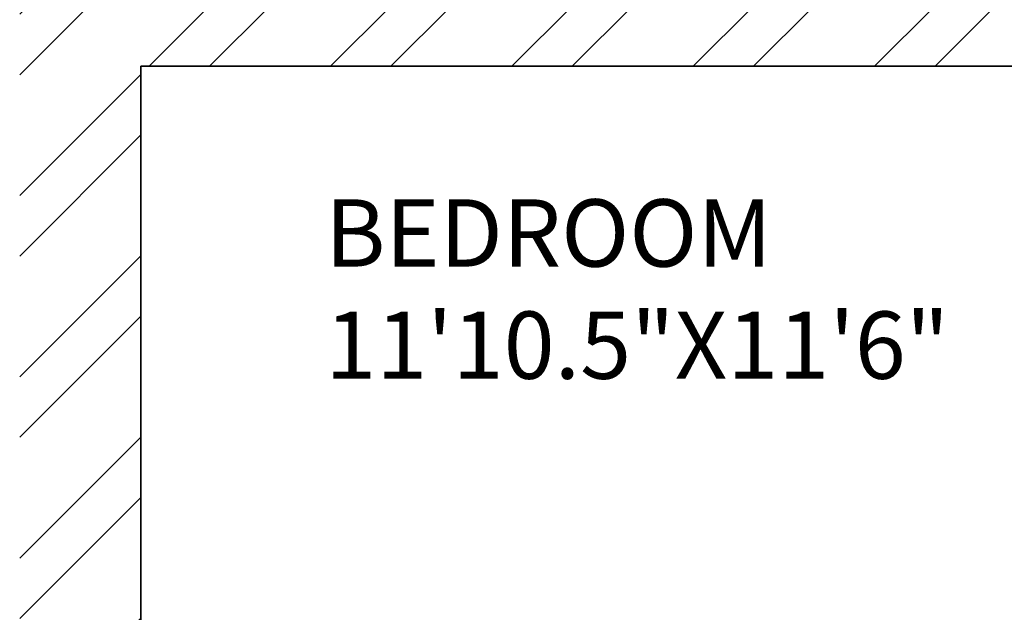
# Model space of a CAD drawing. Units: inches. Extents: x 2120 to 4013, y 1390 to 3019.
# Tile 18 of 59: x 2716 to 2789, y 1688 to 1732. Entities that reach past the tile are written whole.
import ezdxf

# ---------------------------------------------------------------- set-up
doc = ezdxf.new("R2010")
doc.units = ezdxf.units.IN
for name, color, linetype, lineweight in [('A-AREA-IDEN', 7, 'Continuous', 18), ('A-WALL', 7, 'Continuous', 35), ('A-WALL-PATT', 252, 'Continuous', 13)]:
    doc.layers.add(name, color=color, linetype=linetype, lineweight=lineweight)
doc.styles.get("Standard").update_dxf_attribs({"font": 'arial.ttf'})

msp = doc.modelspace()

# ---------------------------------------------------------------- hatches: boundary and pattern name
at = {"layer": 'A-WALL-PATT'}
h = msp.add_hatch(dxfattribs=at)
h.set_pattern_fill('ANSI32', color=256)
h.paths.add_polyline_path([(2271.7331, 2343.531), (2283.3788, 2343.531), (2283.3788, 2348.031), (2283.3788, 2352.5306), (2262.7331, 2352.5306), (2262.7331, 2182.638), (2267.2331, 2182.638), (2271.7331, 2182.638), (2271.7331, 2219.031), (2391.7331, 2219.031), (2391.7331, 2214.189), (2393.9831, 2214.189), (2396.2331, 2214.189), (2396.2331, 2219.031), (2420.2331, 2219.031), (2420.2331, 2225.7535), (2417.2197, 2225.7535), (2415.7331, 2225.7535), (2415.7331, 2223.5306), (2271.7331, 2223.5306)])
h.paths.add_polyline_path([(2380.0942, 2352.5306), (2343.3788, 2352.5306), (2343.3788, 2343.531), (2363.2331, 2343.531), (2363.2331, 2288.8489), (2365.4831, 2288.8489), (2367.7331, 2288.8489), (2367.7331, 2343.531), (2380.0942, 2343.531)], flags=17)
h.paths.add_polyline_path([(2432.4339, 2352.5306), (2404.0943, 2352.5306), (2404.0943, 2343.531), (2415.7331, 2343.531), (2415.7331, 2264.0306), (2367.7331, 2264.0306), (2367.7331, 2266.4872), (2363.2331, 2266.4872), (2363.2331, 2259.531), (2367.7331, 2259.531), (2415.7331, 2259.531), (2415.7331, 2255.0658), (2420.2331, 2255.0658), (2420.2331, 2259.531), (2424.5717, 2259.531), (2424.5717, 2261.781), (2424.5717, 2264.0306), (2420.2331, 2264.0306), (2420.2331, 2343.531), (2432.4339, 2343.531)])
h.paths.add_polyline_path([(2508.9115, 2352.5306), (2456.4339, 2352.5306), (2456.4339, 2343.531), (2468.2331, 2343.531), (2468.2331, 2264.0306), (2448.0487, 2264.0306), (2448.0487, 2259.531), (2468.2331, 2259.531), (2468.2331, 2255.5496), (2472.7331, 2255.5496), (2472.7331, 2343.531), (2508.9115, 2343.531)])
h.paths.add_polyline_path([(2637.7331, 2352.5306), (2544.9116, 2352.5306), (2544.9116, 2343.531), (2589.7331, 2343.531), (2633.2331, 2343.531), (2637.7331, 2343.531)])
h.paths.add_polyline_path([(2594.2331, 2343.5306), (2589.7331, 2343.5306), (2589.7331, 2259.5306), (2589.7331, 2252.4915), (2591.9831, 2252.4915), (2594.2331, 2252.4915)])
h.paths.add_polyline_path([(2637.7331, 2223.5306), (2594.2331, 2223.5306), (2594.2331, 2230.1988), (2591.9831, 2230.1988), (2589.7331, 2230.1988), (2589.7331, 2223.5306), (2472.7331, 2223.5306), (2468.2331, 2223.5306), (2468.2331, 2219.031), (2628.7331, 2219.031), (2628.7331, 2138.031), (2637.7331, 2138.031)])
h.paths.add_polyline_path([(3822.6535, 2458.4402), (3874.9468, 2458.4402), (3874.9468, 2476.9866), (3822.6535, 2476.9866)], flags=9)
h.paths.add_polyline_path([(3834.6921, 2781.8174), (3935.9206, 2781.8174), (3935.9206, 2800.3638), (3834.6921, 2800.3638)], flags=9)
h.paths.add_polyline_path([(3832.2843, 2837.9683), (3884.5776, 2837.9683), (3884.5776, 2856.5146), (3832.2843, 2856.5146)], flags=9)
h.paths.add_polyline_path([(3830.9388, 2861.4782), (3956.8958, 2861.4782), (3956.8958, 2880.0245), (3830.9388, 2880.0245)], flags=9)
h.paths.add_polyline_path([(3870.6966, 2352.5752), (3887.9272, 2352.5752), (3887.9272, 2377.3037), (3870.6966, 2377.3037)], flags=9)
h.paths.add_polyline_path([(3289.2701, 2413.161), (3435.2223, 2413.161), (3435.2223, 2450.2538), (3289.2701, 2450.2538)], flags=9)
h.paths.add_polyline_path([(2487.6944, 2414.3601), (2637.8335, 2414.3601), (2637.8335, 2451.4528), (2487.6944, 2451.4528)], flags=9)
h.paths.add_polyline_path([(2567.3724, 1457.9199), (2815.296, 1457.9199), (2815.296, 1495.0127), (2567.3724, 1495.0127)], flags=9)
h.paths.add_polyline_path([(2655.3825, 2093.2363), (2685.9555, 2093.2363), (2685.9555, 2111.8937), (2655.3825, 2111.8937)], flags=9)
h.paths.add_polyline_path([(2543.9218, 1550.6671), (2587.8406, 1550.6671), (2587.8406, 1569.3244), (2543.9218, 1569.3244)], flags=9)
h.paths.add_polyline_path([(2905.1384, 1543.8113), (2949.0572, 1543.8113), (2949.0572, 1562.4686), (2905.1384, 1562.4686)], flags=9)
h.paths.add_polyline_path([(2736.4118, 1702.4736), (2784.2153, 1702.4736), (2784.2153, 1721.1309), (2736.4118, 1721.1309)], flags=9)
h.paths.add_polyline_path([(2912.8666, 1710.4168), (2951.707, 1710.4168), (2951.707, 1729.0741), (2912.8666, 1729.0741)], flags=9)
h.paths.add_polyline_path([(2923.5785, 1763.5038), (2959.7279, 1763.5038), (2959.7279, 1782.1611), (2923.5785, 1782.1611)], flags=9)
h.paths.add_polyline_path([(2925.2114, 1809.6137), (2967.1861, 1809.6137), (2967.1861, 1828.271), (2925.2114, 1828.271)], flags=9)
h.paths.add_polyline_path([(2996.2711, 1878.9003), (2996.2711, 1913.109), (2977.6138, 1913.109), (2977.6138, 1878.9003)], flags=9)
h.paths.add_polyline_path([(2883.0859, 1895.7192), (2927.1855, 1895.7192), (2927.1855, 1914.3766), (2883.0859, 1914.3766)], flags=9)
h.paths.add_polyline_path([(2787.3924, 1810.8013), (2841.0213, 1810.8013), (2841.0213, 1829.4587), (2787.3924, 1829.4587)], flags=9)
h.paths.add_polyline_path([(2775.6399, 2101.7395), (2829.2689, 2101.7395), (2829.2689, 2120.3968), (2775.6399, 2120.3968)], flags=9)
h.paths.add_polyline_path([(2913.0263, 2075.817), (2951.8667, 2075.817), (2951.8667, 2094.4744), (2913.0263, 2094.4744)], flags=9)
h.paths.add_polyline_path([(2929.966, 2133.3669), (2966.1154, 2133.3669), (2966.1154, 2152.0243), (2929.966, 2152.0243)], flags=9)
h.paths.add_polyline_path([(2932.7502, 2182.6088), (2968.8996, 2182.6088), (2968.8996, 2201.2662), (2932.7502, 2201.2662)], flags=9)
h.paths.add_polyline_path([(2996.0681, 2266.3173), (2996.0681, 2300.5261), (2977.4108, 2300.5261), (2977.4108, 2266.3173)], flags=9)
h.paths.add_polyline_path([(2885.1039, 2279.2186), (2929.2035, 2279.2186), (2929.2035, 2297.8759), (2885.1039, 2297.8759)], flags=9)
h.paths.add_polyline_path([(2735.7042, 2218.3197), (2783.5078, 2218.3197), (2783.5078, 2236.9771), (2735.7042, 2236.9771)], flags=9)
h.paths.add_polyline_path([(2635.6049, 2044.0085), (2648.9678, 2044.0085), (2648.9678, 2054.312), (2635.6049, 2054.312)], flags=9)
h.paths.add_polyline_path([(2714.0148, 1923.0473), (2727.3777, 1923.0473), (2727.3777, 1933.3508), (2714.0148, 1933.3508)], flags=9)
h.paths.add_polyline_path([(2709.0345, 1988.1628), (2722.3974, 1988.1628), (2722.3974, 1998.4663), (2709.0345, 1998.4663)], flags=9)
h.paths.add_polyline_path([(2592.8935, 1962.1763), (2606.2564, 1962.1763), (2606.2564, 1972.4799), (2592.8935, 1972.4799)], flags=9)
h.paths.add_polyline_path([(2618.3996, 1985.9724), (2644.1942, 1985.9724), (2644.1942, 1996.2759), (2618.3996, 1996.2759)], flags=9)
h.paths.add_polyline_path([(2601.279, 1920.5869), (2614.6419, 1920.5869), (2614.6419, 1930.8904), (2601.279, 1930.8904)], flags=9)
h.paths.add_polyline_path([(2692.3278, 1932.7645), (2704.5311, 1932.7645), (2704.5311, 1943.0681), (2692.3278, 1943.0681)], flags=9)
h.paths.add_polyline_path([(2311.122, 1672.7318), (2355.0408, 1672.7318), (2355.0408, 1691.3892), (2311.122, 1691.3892)], flags=9)
h.paths.add_polyline_path([(2456.2551, 1632.3198), (2492.4796, 1632.3198), (2492.4796, 1650.9772), (2456.2551, 1650.9772)], flags=9)
h.paths.add_polyline_path([(2401.0766, 1631.4793), (2437.301, 1631.4793), (2437.301, 1650.1367), (2401.0766, 1650.1367)], flags=9)
h.paths.add_polyline_path([(2546.7054, 1700.9235), (2594.509, 1700.9235), (2594.509, 1719.5809), (2546.7054, 1719.5809)], flags=9)
h.paths.add_polyline_path([(2445.4866, 1766.9937), (2497.5261, 1766.9937), (2497.5261, 1785.651), (2445.4866, 1785.651)], flags=9)
h.paths.add_polyline_path([(2287.9992, 1739.7675), (2326.8396, 1739.7675), (2326.8396, 1758.4248), (2287.9992, 1758.4248)], flags=9)
h.paths.add_polyline_path([(2458.5279, 1924.7607), (2510.5675, 1924.7607), (2510.5675, 1943.4181), (2458.5279, 1943.4181)], flags=9)
h.paths.add_polyline_path([(2309.2811, 1902.7642), (2345.4305, 1902.7642), (2345.4305, 1921.4215), (2309.2811, 1921.4215)], flags=9)
h.paths.add_polyline_path([(2490.7554, 2018.9392), (2530.7896, 2018.9392), (2530.7896, 2037.5965), (2490.7554, 2037.5965)], flags=9)
h.paths.add_polyline_path([(2402.143, 2024.7393), (2438.5414, 2024.7393), (2438.5414, 2043.3966), (2402.143, 2043.3966)], flags=9)
h.paths.add_polyline_path([(2287.856, 1931.7926), (2326.6964, 1931.7926), (2326.6964, 1950.4499), (2287.856, 1950.4499)], flags=9)
h.paths.add_polyline_path([(2281.7979, 2193.5771), (2320.6383, 2193.5771), (2320.6383, 2212.2344), (2281.7979, 2212.2344)], flags=25)
h.paths.add_polyline_path([(2484.0754, 2093.892), (2536.115, 2093.892), (2536.115, 2112.5494), (2484.0754, 2112.5494)], flags=9)
h.paths.add_polyline_path([(2624.7948, 2281.8639), (2624.7948, 2311.4137), (2606.1375, 2311.4137), (2606.1375, 2281.8639)], flags=9)
h.paths.add_polyline_path([(2507.5036, 2290.3639), (2541.934, 2290.3639), (2541.934, 2309.0212), (2507.5036, 2309.0212)], flags=9)
h.paths.add_polyline_path([(2423.1076, 2285.2202), (2459.332, 2285.2202), (2459.332, 2303.8776), (2423.1076, 2303.8776)], flags=9)
h.paths.add_polyline_path([(2374.5467, 2289.6272), (2410.7711, 2289.6272), (2410.7711, 2308.2846), (2374.5467, 2308.2846)], flags=25)
h.paths.add_polyline_path([(2277.4907, 2227.5651), (2316.3311, 2227.5651), (2316.3311, 2246.2224), (2277.4907, 2246.2224)], flags=25)
h.paths.add_polyline_path([(2655.3825, 2093.2367), (2685.9555, 2093.2367), (2685.9555, 2111.894), (2655.3825, 2111.894)], flags=9)
h.paths.add_polyline_path([(2543.9217, 1550.6674), (2587.8406, 1550.6674), (2587.8406, 1569.3247), (2543.9217, 1569.3247)], flags=9)
h.paths.add_polyline_path([(2905.1384, 1543.8116), (2949.0572, 1543.8116), (2949.0572, 1562.4689), (2905.1384, 1562.4689)], flags=9)
h.paths.add_polyline_path([(2736.4118, 1702.4739), (2784.2153, 1702.4739), (2784.2153, 1721.1312), (2736.4118, 1721.1312)], flags=9)
h.paths.add_polyline_path([(2912.8666, 1710.4171), (2951.707, 1710.4171), (2951.707, 1729.0744), (2912.8666, 1729.0744)], flags=9)
h.paths.add_polyline_path([(2923.5785, 1763.5041), (2959.7279, 1763.5041), (2959.7279, 1782.1614), (2923.5785, 1782.1614)], flags=9)
h.paths.add_polyline_path([(2925.2114, 1809.614), (2967.1861, 1809.614), (2967.1861, 1828.2713), (2925.2114, 1828.2713)], flags=9)
h.paths.add_polyline_path([(2996.2711, 1878.9006), (2996.2711, 1913.1094), (2977.6137, 1913.1094), (2977.6137, 1878.9006)], flags=9)
h.paths.add_polyline_path([(2883.0859, 1895.7195), (2927.1855, 1895.7195), (2927.1855, 1914.3769), (2883.0859, 1914.3769)], flags=9)
h.paths.add_polyline_path([(2787.3924, 1810.8016), (2841.0213, 1810.8016), (2841.0213, 1829.459), (2787.3924, 1829.459)], flags=9)
h.paths.add_polyline_path([(2775.6399, 2101.7398), (2829.2688, 2101.7398), (2829.2688, 2120.3971), (2775.6399, 2120.3971)], flags=9)
h.paths.add_polyline_path([(2913.0263, 2075.8173), (2951.8667, 2075.8173), (2951.8667, 2094.4747), (2913.0263, 2094.4747)], flags=9)
h.paths.add_polyline_path([(2929.966, 2133.3672), (2966.1154, 2133.3672), (2966.1154, 2152.0246), (2929.966, 2152.0246)], flags=9)
h.paths.add_polyline_path([(2932.7502, 2182.6091), (2968.8996, 2182.6091), (2968.8996, 2201.2665), (2932.7502, 2201.2665)], flags=9)
h.paths.add_polyline_path([(2996.0681, 2266.3176), (2996.0681, 2300.5264), (2977.4108, 2300.5264), (2977.4108, 2266.3176)], flags=9)
h.paths.add_polyline_path([(2885.1039, 2279.2189), (2929.2035, 2279.2189), (2929.2035, 2297.8762), (2885.1039, 2297.8762)], flags=9)
h.paths.add_polyline_path([(2735.7042, 2218.32), (2783.5078, 2218.32), (2783.5078, 2236.9774), (2735.7042, 2236.9774)], flags=9)
h.paths.add_polyline_path([(2635.6048, 2044.0088), (2648.9677, 2044.0088), (2648.9677, 2054.3123), (2635.6048, 2054.3123)], flags=9)
h.paths.add_polyline_path([(2714.0148, 1923.0476), (2727.3777, 1923.0476), (2727.3777, 1933.3511), (2714.0148, 1933.3511)], flags=9)
h.paths.add_polyline_path([(2709.0345, 1988.1631), (2722.3974, 1988.1631), (2722.3974, 1998.4666), (2709.0345, 1998.4666)], flags=9)
h.paths.add_polyline_path([(2592.8935, 1962.1766), (2606.2564, 1962.1766), (2606.2564, 1972.4802), (2592.8935, 1972.4802)], flags=9)
h.paths.add_polyline_path([(2618.3995, 1985.9727), (2644.1942, 1985.9727), (2644.1942, 1996.2762), (2618.3995, 1996.2762)], flags=9)
h.paths.add_polyline_path([(2601.279, 1920.5872), (2614.6419, 1920.5872), (2614.6419, 1930.8908), (2601.279, 1930.8908)], flags=9)
h.paths.add_polyline_path([(2692.3278, 1932.7648), (2704.5311, 1932.7648), (2704.5311, 1943.0684), (2692.3278, 1943.0684)], flags=9)
h.paths.add_polyline_path([(2311.122, 1672.7321), (2355.0408, 1672.7321), (2355.0408, 1691.3895), (2311.122, 1691.3895)], flags=9)
h.paths.add_polyline_path([(2456.2551, 1632.3201), (2492.4795, 1632.3201), (2492.4795, 1650.9775), (2456.2551, 1650.9775)], flags=9)
h.paths.add_polyline_path([(2401.0766, 1631.4796), (2437.301, 1631.4796), (2437.301, 1650.137), (2401.0766, 1650.137)], flags=9)
h.paths.add_polyline_path([(2546.7054, 1700.9238), (2594.509, 1700.9238), (2594.509, 1719.5812), (2546.7054, 1719.5812)], flags=9)
h.paths.add_polyline_path([(2445.4866, 1766.994), (2497.5261, 1766.994), (2497.5261, 1785.6513), (2445.4866, 1785.6513)], flags=9)
h.paths.add_polyline_path([(2287.9992, 1739.7678), (2326.8396, 1739.7678), (2326.8396, 1758.4251), (2287.9992, 1758.4251)], flags=9)
h.paths.add_polyline_path([(2458.5279, 1924.7611), (2510.5675, 1924.7611), (2510.5675, 1943.4184), (2458.5279, 1943.4184)], flags=9)
h.paths.add_polyline_path([(2309.2811, 1902.7645), (2345.4305, 1902.7645), (2345.4305, 1921.4218), (2309.2811, 1921.4218)], flags=9)
h.paths.add_polyline_path([(2490.7554, 2018.9395), (2530.7895, 2018.9395), (2530.7895, 2037.5968), (2490.7554, 2037.5968)], flags=9)
h.paths.add_polyline_path([(2402.143, 2024.7396), (2438.5413, 2024.7396), (2438.5413, 2043.3969), (2402.143, 2043.3969)], flags=9)
h.paths.add_polyline_path([(2287.856, 1931.7929), (2326.6964, 1931.7929), (2326.6964, 1950.4502), (2287.856, 1950.4502)], flags=9)
h.paths.add_polyline_path([(2281.7979, 2193.5774), (2320.6383, 2193.5774), (2320.6383, 2212.2347), (2281.7979, 2212.2347)], flags=25)
h.paths.add_polyline_path([(2484.0754, 2093.8924), (2536.115, 2093.8924), (2536.115, 2112.5497), (2484.0754, 2112.5497)], flags=9)
h.paths.add_polyline_path([(2624.7948, 2281.8642), (2624.7948, 2311.414), (2606.1374, 2311.414), (2606.1374, 2281.8642)], flags=9)
h.paths.add_polyline_path([(2507.5035, 2290.3642), (2541.934, 2290.3642), (2541.934, 2309.0215), (2507.5035, 2309.0215)], flags=9)
h.paths.add_polyline_path([(2423.1075, 2285.2205), (2459.332, 2285.2205), (2459.332, 2303.8779), (2423.1075, 2303.8779)], flags=9)
h.paths.add_polyline_path([(2374.5467, 2289.6275), (2410.7711, 2289.6275), (2410.7711, 2308.2849), (2374.5467, 2308.2849)], flags=25)
h.paths.add_polyline_path([(2277.4907, 2227.5654), (2316.3311, 2227.5654), (2316.3311, 2246.2227), (2277.4907, 2246.2227)], flags=25)
h = msp.add_hatch(dxfattribs=at)
h.set_pattern_fill('ANSI32', color=256)
h.paths.add_polyline_path([(2271.7331, 1980.389), (2262.7331, 1980.389), (2262.7331, 1912.8434), (2267.2331, 1912.8434), (2271.7331, 1912.8434), (2271.7331, 1922.531), (2351.2331, 1922.531), (2351.2331, 1901.4728), (2355.7331, 1901.4728), (2355.7331, 1922.531), (2357.9815, 1922.531), (2357.9815, 1926.5306), (2271.7331, 1926.5306)])
h.paths.add_polyline_path([(2589.2331, 1949.1622), (2584.7331, 1949.1622), (2580.2331, 1949.1622), (2580.2331, 1874.5306), (2355.7331, 1874.5306), (2355.7331, 1880.1922), (2351.2331, 1880.1922), (2351.2331, 1874.5306), (2271.7331, 1874.5306), (2271.7331, 1888.8431), (2262.7331, 1888.8431), (2262.7331, 1842.2909), (2267.2331, 1842.2909), (2271.7331, 1842.2909), (2271.7331, 1865.531), (2415.7331, 1865.531), (2415.7331, 1779.7286), (2420.2331, 1779.7286), (2420.2331, 1865.531), (2589.2331, 1865.531)])
h.paths.add_polyline_path([(2271.7331, 1782.2906), (2262.7331, 1782.2906), (2262.7331, 1711.4639), (2267.2331, 1711.4639), (2271.7331, 1711.4639), (2271.7331, 1738.031), (2420.2331, 1738.031), (2420.2331, 1742.531), (2420.2331, 1747.3376), (2417.9831, 1747.3376), (2415.7331, 1747.3376), (2415.7331, 1742.5306), (2271.7331, 1742.5306)])
h.paths.add_polyline_path([(2271.7331, 1627.031), (2362.3957, 1627.031), (2362.3957, 1629.281), (2362.3957, 1631.5306), (2271.7331, 1631.5306), (2271.7331, 1675.4636), (2262.7331, 1675.4636), (2262.7331, 1581.531), (2405.3032, 1581.531), (2405.3032, 1586.031), (2405.3032, 1590.5306), (2396.2331, 1590.5306), (2396.2331, 1691.4513), (2418.7206, 1691.4513), (2418.7206, 1695.951), (2396.2331, 1695.951), (2391.7331, 1695.951), (2391.7331, 1631.5306), (2386.7425, 1631.5306), (2386.7425, 1629.2806), (2386.7425, 1627.031), (2391.7331, 1627.031), (2391.7331, 1586.1709), (2271.7331, 1586.1709)])
h.paths.add_polyline_path([(2459.6703, 1590.5306), (2429.3032, 1590.5306), (2429.3032, 1581.531), (2459.6703, 1581.531), (2459.6703, 1586.031)])
h.paths.add_polyline_path([(2501.2331, 1590.531), (2501.2331, 1665.0195), (2498.9831, 1665.0195), (2496.7331, 1665.0195), (2496.7331, 1590.5306), (2483.8201, 1590.5306), (2483.8201, 1590.1579), (2483.6704, 1590.1579), (2483.6704, 1581.531), (2505.0196, 1581.531), (2505.0196, 1583.781), (2505.0196, 1586.0306), (2501.2331, 1586.0306)])
h.paths.add_polyline_path([(2544.1361, 1583.781), (2544.1361, 1586.0306), (2527.1368, 1586.0306), (2527.1368, 1583.7806), (2527.1368, 1581.531), (2544.1361, 1581.531)])
h.paths.add_polyline_path([(3822.6535, 2458.4402), (3874.9468, 2458.4402), (3874.9468, 2476.9866), (3822.6535, 2476.9866)], flags=9)
h.paths.add_polyline_path([(3834.6921, 2781.8174), (3935.9206, 2781.8174), (3935.9206, 2800.3638), (3834.6921, 2800.3638)], flags=9)
h.paths.add_polyline_path([(3832.2843, 2837.9683), (3884.5776, 2837.9683), (3884.5776, 2856.5146), (3832.2843, 2856.5146)], flags=9)
h.paths.add_polyline_path([(3830.9388, 2861.4782), (3956.8958, 2861.4782), (3956.8958, 2880.0245), (3830.9388, 2880.0245)], flags=9)
h.paths.add_polyline_path([(3870.6966, 2352.5752), (3887.9272, 2352.5752), (3887.9272, 2377.3037), (3870.6966, 2377.3037)], flags=9)
h.paths.add_polyline_path([(3289.2701, 2413.161), (3435.2223, 2413.161), (3435.2223, 2450.2538), (3289.2701, 2450.2538)], flags=9)
h.paths.add_polyline_path([(2487.6944, 2414.3601), (2637.8335, 2414.3601), (2637.8335, 2451.4528), (2487.6944, 2451.4528)], flags=9)
h.paths.add_polyline_path([(2567.3724, 1457.9199), (2815.296, 1457.9199), (2815.296, 1495.0127), (2567.3724, 1495.0127)], flags=9)
h.paths.add_polyline_path([(2655.3825, 2093.2363), (2685.9555, 2093.2363), (2685.9555, 2111.8937), (2655.3825, 2111.8937)], flags=9)
h.paths.add_polyline_path([(2543.9218, 1550.6671), (2587.8406, 1550.6671), (2587.8406, 1569.3244), (2543.9218, 1569.3244)], flags=9)
h.paths.add_polyline_path([(2905.1384, 1543.8113), (2949.0572, 1543.8113), (2949.0572, 1562.4686), (2905.1384, 1562.4686)], flags=9)
h.paths.add_polyline_path([(2736.4118, 1702.4736), (2784.2153, 1702.4736), (2784.2153, 1721.1309), (2736.4118, 1721.1309)], flags=9)
h.paths.add_polyline_path([(2912.8666, 1710.4168), (2951.707, 1710.4168), (2951.707, 1729.0741), (2912.8666, 1729.0741)], flags=9)
h.paths.add_polyline_path([(2923.5785, 1763.5038), (2959.7279, 1763.5038), (2959.7279, 1782.1611), (2923.5785, 1782.1611)], flags=9)
h.paths.add_polyline_path([(2925.2114, 1809.6137), (2967.1861, 1809.6137), (2967.1861, 1828.271), (2925.2114, 1828.271)], flags=9)
h.paths.add_polyline_path([(2996.2711, 1878.9003), (2996.2711, 1913.109), (2977.6138, 1913.109), (2977.6138, 1878.9003)], flags=9)
h.paths.add_polyline_path([(2883.0859, 1895.7192), (2927.1855, 1895.7192), (2927.1855, 1914.3766), (2883.0859, 1914.3766)], flags=9)
h.paths.add_polyline_path([(2787.3924, 1810.8013), (2841.0213, 1810.8013), (2841.0213, 1829.4587), (2787.3924, 1829.4587)], flags=9)
h.paths.add_polyline_path([(2775.6399, 2101.7395), (2829.2689, 2101.7395), (2829.2689, 2120.3968), (2775.6399, 2120.3968)], flags=9)
h.paths.add_polyline_path([(2913.0263, 2075.817), (2951.8667, 2075.817), (2951.8667, 2094.4744), (2913.0263, 2094.4744)], flags=9)
h.paths.add_polyline_path([(2929.966, 2133.3669), (2966.1154, 2133.3669), (2966.1154, 2152.0243), (2929.966, 2152.0243)], flags=9)
h.paths.add_polyline_path([(2932.7502, 2182.6088), (2968.8996, 2182.6088), (2968.8996, 2201.2662), (2932.7502, 2201.2662)], flags=9)
h.paths.add_polyline_path([(2996.0681, 2266.3173), (2996.0681, 2300.5261), (2977.4108, 2300.5261), (2977.4108, 2266.3173)], flags=9)
h.paths.add_polyline_path([(2885.1039, 2279.2186), (2929.2035, 2279.2186), (2929.2035, 2297.8759), (2885.1039, 2297.8759)], flags=9)
h.paths.add_polyline_path([(2735.7042, 2218.3197), (2783.5078, 2218.3197), (2783.5078, 2236.9771), (2735.7042, 2236.9771)], flags=9)
h.paths.add_polyline_path([(2635.6049, 2044.0085), (2648.9678, 2044.0085), (2648.9678, 2054.312), (2635.6049, 2054.312)], flags=9)
h.paths.add_polyline_path([(2714.0148, 1923.0473), (2727.3777, 1923.0473), (2727.3777, 1933.3508), (2714.0148, 1933.3508)], flags=9)
h.paths.add_polyline_path([(2709.0345, 1988.1628), (2722.3974, 1988.1628), (2722.3974, 1998.4663), (2709.0345, 1998.4663)], flags=9)
h.paths.add_polyline_path([(2592.8935, 1962.1763), (2606.2564, 1962.1763), (2606.2564, 1972.4799), (2592.8935, 1972.4799)], flags=9)
h.paths.add_polyline_path([(2618.3996, 1985.9724), (2644.1942, 1985.9724), (2644.1942, 1996.2759), (2618.3996, 1996.2759)], flags=9)
h.paths.add_polyline_path([(2601.279, 1920.5869), (2614.6419, 1920.5869), (2614.6419, 1930.8904), (2601.279, 1930.8904)], flags=9)
h.paths.add_polyline_path([(2692.3278, 1932.7645), (2704.5311, 1932.7645), (2704.5311, 1943.0681), (2692.3278, 1943.0681)], flags=9)
h.paths.add_polyline_path([(2311.122, 1672.7318), (2355.0408, 1672.7318), (2355.0408, 1691.3892), (2311.122, 1691.3892)], flags=25)
h.paths.add_polyline_path([(2456.2551, 1632.3198), (2492.4796, 1632.3198), (2492.4796, 1650.9772), (2456.2551, 1650.9772)], flags=9)
h.paths.add_polyline_path([(2401.0766, 1631.4793), (2437.301, 1631.4793), (2437.301, 1650.1367), (2401.0766, 1650.1367)], flags=9)
h.paths.add_polyline_path([(2546.7054, 1700.9235), (2594.509, 1700.9235), (2594.509, 1719.5809), (2546.7054, 1719.5809)], flags=9)
h.paths.add_polyline_path([(2445.4866, 1766.9937), (2497.5261, 1766.9937), (2497.5261, 1785.651), (2445.4866, 1785.651)], flags=9)
h.paths.add_polyline_path([(2287.9992, 1739.7675), (2326.8396, 1739.7675), (2326.8396, 1758.4248), (2287.9992, 1758.4248)], flags=24)
h.paths.add_polyline_path([(2458.5279, 1924.7607), (2510.5675, 1924.7607), (2510.5675, 1943.4181), (2458.5279, 1943.4181)], flags=25)
h.paths.add_polyline_path([(2309.2811, 1902.7642), (2345.4305, 1902.7642), (2345.4305, 1921.4215), (2309.2811, 1921.4215)], flags=25)
h.paths.add_polyline_path([(2490.7554, 2018.9392), (2530.7896, 2018.9392), (2530.7896, 2037.5965), (2490.7554, 2037.5965)], flags=9)
h.paths.add_polyline_path([(2402.143, 2024.7393), (2438.5414, 2024.7393), (2438.5414, 2043.3966), (2402.143, 2043.3966)], flags=9)
h.paths.add_polyline_path([(2287.856, 1931.7926), (2326.6964, 1931.7926), (2326.6964, 1950.4499), (2287.856, 1950.4499)], flags=25)
h.paths.add_polyline_path([(2281.7979, 2193.5771), (2320.6383, 2193.5771), (2320.6383, 2212.2344), (2281.7979, 2212.2344)], flags=9)
h.paths.add_polyline_path([(2484.0754, 2093.892), (2536.115, 2093.892), (2536.115, 2112.5494), (2484.0754, 2112.5494)], flags=9)
h.paths.add_polyline_path([(2624.7948, 2281.8639), (2624.7948, 2311.4137), (2606.1375, 2311.4137), (2606.1375, 2281.8639)], flags=9)
h.paths.add_polyline_path([(2507.5036, 2290.3639), (2541.934, 2290.3639), (2541.934, 2309.0212), (2507.5036, 2309.0212)], flags=9)
h.paths.add_polyline_path([(2423.1076, 2285.2202), (2459.332, 2285.2202), (2459.332, 2303.8776), (2423.1076, 2303.8776)], flags=9)
h.paths.add_polyline_path([(2374.5467, 2289.6272), (2410.7711, 2289.6272), (2410.7711, 2308.2846), (2374.5467, 2308.2846)], flags=9)
h.paths.add_polyline_path([(2277.4907, 2227.5651), (2316.3311, 2227.5651), (2316.3311, 2246.2224), (2277.4907, 2246.2224)], flags=9)
h.paths.add_polyline_path([(2655.3825, 2093.2367), (2685.9555, 2093.2367), (2685.9555, 2111.894), (2655.3825, 2111.894)], flags=9)
h.paths.add_polyline_path([(2543.9217, 1550.6674), (2587.8406, 1550.6674), (2587.8406, 1569.3247), (2543.9217, 1569.3247)], flags=9)
h.paths.add_polyline_path([(2905.1384, 1543.8116), (2949.0572, 1543.8116), (2949.0572, 1562.4689), (2905.1384, 1562.4689)], flags=9)
h.paths.add_polyline_path([(2736.4118, 1702.4739), (2784.2153, 1702.4739), (2784.2153, 1721.1312), (2736.4118, 1721.1312)], flags=9)
h.paths.add_polyline_path([(2912.8666, 1710.4171), (2951.707, 1710.4171), (2951.707, 1729.0744), (2912.8666, 1729.0744)], flags=9)
h.paths.add_polyline_path([(2923.5785, 1763.5041), (2959.7279, 1763.5041), (2959.7279, 1782.1614), (2923.5785, 1782.1614)], flags=9)
h.paths.add_polyline_path([(2925.2114, 1809.614), (2967.1861, 1809.614), (2967.1861, 1828.2713), (2925.2114, 1828.2713)], flags=9)
h.paths.add_polyline_path([(2996.2711, 1878.9006), (2996.2711, 1913.1094), (2977.6137, 1913.1094), (2977.6137, 1878.9006)], flags=9)
h.paths.add_polyline_path([(2883.0859, 1895.7195), (2927.1855, 1895.7195), (2927.1855, 1914.3769), (2883.0859, 1914.3769)], flags=9)
h.paths.add_polyline_path([(2787.3924, 1810.8016), (2841.0213, 1810.8016), (2841.0213, 1829.459), (2787.3924, 1829.459)], flags=9)
h.paths.add_polyline_path([(2775.6399, 2101.7398), (2829.2688, 2101.7398), (2829.2688, 2120.3971), (2775.6399, 2120.3971)], flags=9)
h.paths.add_polyline_path([(2913.0263, 2075.8173), (2951.8667, 2075.8173), (2951.8667, 2094.4747), (2913.0263, 2094.4747)], flags=9)
h.paths.add_polyline_path([(2929.966, 2133.3672), (2966.1154, 2133.3672), (2966.1154, 2152.0246), (2929.966, 2152.0246)], flags=9)
h.paths.add_polyline_path([(2932.7502, 2182.6091), (2968.8996, 2182.6091), (2968.8996, 2201.2665), (2932.7502, 2201.2665)], flags=9)
h.paths.add_polyline_path([(2996.0681, 2266.3176), (2996.0681, 2300.5264), (2977.4108, 2300.5264), (2977.4108, 2266.3176)], flags=9)
h.paths.add_polyline_path([(2885.1039, 2279.2189), (2929.2035, 2279.2189), (2929.2035, 2297.8762), (2885.1039, 2297.8762)], flags=9)
h.paths.add_polyline_path([(2735.7042, 2218.32), (2783.5078, 2218.32), (2783.5078, 2236.9774), (2735.7042, 2236.9774)], flags=9)
h.paths.add_polyline_path([(2635.6048, 2044.0088), (2648.9677, 2044.0088), (2648.9677, 2054.3123), (2635.6048, 2054.3123)], flags=9)
h.paths.add_polyline_path([(2714.0148, 1923.0476), (2727.3777, 1923.0476), (2727.3777, 1933.3511), (2714.0148, 1933.3511)], flags=9)
h.paths.add_polyline_path([(2709.0345, 1988.1631), (2722.3974, 1988.1631), (2722.3974, 1998.4666), (2709.0345, 1998.4666)], flags=9)
h.paths.add_polyline_path([(2592.8935, 1962.1766), (2606.2564, 1962.1766), (2606.2564, 1972.4802), (2592.8935, 1972.4802)], flags=9)
h.paths.add_polyline_path([(2618.3995, 1985.9727), (2644.1942, 1985.9727), (2644.1942, 1996.2762), (2618.3995, 1996.2762)], flags=9)
h.paths.add_polyline_path([(2601.279, 1920.5872), (2614.6419, 1920.5872), (2614.6419, 1930.8908), (2601.279, 1930.8908)], flags=9)
h.paths.add_polyline_path([(2692.3278, 1932.7648), (2704.5311, 1932.7648), (2704.5311, 1943.0684), (2692.3278, 1943.0684)], flags=9)
h.paths.add_polyline_path([(2311.122, 1672.7321), (2355.0408, 1672.7321), (2355.0408, 1691.3895), (2311.122, 1691.3895)], flags=25)
h.paths.add_polyline_path([(2456.2551, 1632.3201), (2492.4795, 1632.3201), (2492.4795, 1650.9775), (2456.2551, 1650.9775)], flags=9)
h.paths.add_polyline_path([(2401.0766, 1631.4796), (2437.301, 1631.4796), (2437.301, 1650.137), (2401.0766, 1650.137)], flags=9)
h.paths.add_polyline_path([(2546.7054, 1700.9238), (2594.509, 1700.9238), (2594.509, 1719.5812), (2546.7054, 1719.5812)], flags=9)
h.paths.add_polyline_path([(2445.4866, 1766.994), (2497.5261, 1766.994), (2497.5261, 1785.6513), (2445.4866, 1785.6513)], flags=9)
h.paths.add_polyline_path([(2287.9992, 1739.7678), (2326.8396, 1739.7678), (2326.8396, 1758.4251), (2287.9992, 1758.4251)], flags=24)
h.paths.add_polyline_path([(2458.5279, 1924.7611), (2510.5675, 1924.7611), (2510.5675, 1943.4184), (2458.5279, 1943.4184)], flags=25)
h.paths.add_polyline_path([(2309.2811, 1902.7645), (2345.4305, 1902.7645), (2345.4305, 1921.4218), (2309.2811, 1921.4218)], flags=25)
h.paths.add_polyline_path([(2490.7554, 2018.9395), (2530.7895, 2018.9395), (2530.7895, 2037.5968), (2490.7554, 2037.5968)], flags=9)
h.paths.add_polyline_path([(2402.143, 2024.7396), (2438.5413, 2024.7396), (2438.5413, 2043.3969), (2402.143, 2043.3969)], flags=9)
h.paths.add_polyline_path([(2287.856, 1931.7929), (2326.6964, 1931.7929), (2326.6964, 1950.4502), (2287.856, 1950.4502)], flags=25)
h.paths.add_polyline_path([(2281.7979, 2193.5774), (2320.6383, 2193.5774), (2320.6383, 2212.2347), (2281.7979, 2212.2347)], flags=9)
h.paths.add_polyline_path([(2484.0754, 2093.8924), (2536.115, 2093.8924), (2536.115, 2112.5497), (2484.0754, 2112.5497)], flags=9)
h.paths.add_polyline_path([(2624.7948, 2281.8642), (2624.7948, 2311.414), (2606.1374, 2311.414), (2606.1374, 2281.8642)], flags=9)
h.paths.add_polyline_path([(2507.5035, 2290.3642), (2541.934, 2290.3642), (2541.934, 2309.0215), (2507.5035, 2309.0215)], flags=9)
h.paths.add_polyline_path([(2423.1075, 2285.2205), (2459.332, 2285.2205), (2459.332, 2303.8779), (2423.1075, 2303.8779)], flags=9)
h.paths.add_polyline_path([(2374.5467, 2289.6275), (2410.7711, 2289.6275), (2410.7711, 2308.2849), (2374.5467, 2308.2849)], flags=9)
h.paths.add_polyline_path([(2277.4907, 2227.5654), (2316.3311, 2227.5654), (2316.3311, 2246.2227), (2277.4907, 2246.2227)], flags=9)
h = msp.add_hatch(dxfattribs=at)
h.set_pattern_fill('ANSI32', color=256)
h.paths.add_polyline_path([(2271.7331, 2122.6377), (2262.7331, 2122.6377), (2262.7331, 2040.3893), (2267.2331, 2040.3893), (2271.7331, 2040.3893), (2271.7331, 2044.8856), (2271.7331, 2070.531), (2391.7331, 2070.531), (2391.7331, 1926.5306), (2388.3993, 1926.5306), (2388.3993, 1922.531), (2395.7331, 1922.531), (2395.7331, 1992.531), (2400.4511, 1992.531), (2400.4511, 1997.0306), (2395.7331, 1997.0306), (2395.7331, 2070.531), (2443.7331, 2070.531), (2443.7331, 2046.1368), (2448.2331, 2046.1368), (2448.2331, 2070.531), (2580.2331, 2070.531), (2580.2331, 1997.0306), (2492.9076, 1997.0306), (2492.9076, 1992.531), (2580.2331, 1992.531), (2580.2331, 1983.9368), (2589.2331, 1983.9368), (2589.2331, 2070.531), (2589.2331, 2075.0306), (2396.2331, 2075.0306), (2396.2331, 2184.3565), (2393.9831, 2184.3565), (2391.7331, 2184.3565), (2391.7331, 2075.0306), (2271.7331, 2075.0306)])
h.paths.add_polyline_path([(2724.7331, 2138.0306), (2628.7331, 2138.0306), (2628.7331, 2070.5306), (2628.7331, 2067.0987), (2633.2331, 2067.0987), (2637.7331, 2067.0987), (2637.7331, 2070.531), (2657.3413, 2070.531), (2657.3413, 2079.5306), (2637.7331, 2079.5306), (2637.7331, 2129.031), (2715.7331, 2129.031), (2715.7331, 2079.5306), (2698.0378, 2079.5306), (2698.0378, 2070.531), (2715.7331, 2070.531), (2715.7331, 2012.1531), (2720.2331, 2012.1531), (2724.7331, 2012.1531)])
h.paths.add_polyline_path([(2724.7331, 2213.031), (2831.3209, 2213.031), (2831.3209, 2215.281), (2831.3209, 2217.5306), (2724.7331, 2217.5306), (2724.7331, 2343.531), (2751.8755, 2343.531), (2751.8755, 2352.5306), (2715.7331, 2352.5306), (2715.7331, 2138.031), (2724.7331, 2138.031)])
h.paths.add_polyline_path([(2902.53, 2352.5306), (2811.8755, 2352.5306), (2811.8755, 2343.531), (2867.2331, 2343.531), (2867.2331, 2217.5306), (2863.6364, 2217.5306), (2863.6364, 2213.031), (2871.7331, 2213.031), (2871.7331, 2217.531), (2871.7331, 2343.531), (2902.53, 2343.531)])
h.paths.add_polyline_path([(3009.7331, 2352.5306), (2938.53, 2352.5306), (2938.53, 2343.531), (2966.2331, 2343.531), (2966.2331, 2242.3281), (2968.4831, 2242.3281), (2970.7331, 2242.3281), (2970.7331, 2343.531), (3009.7331, 2343.531)])
h.paths.add_polyline_path([(3009.7331, 2217.5306), (2970.7331, 2217.5306), (2970.7331, 2220.5422), (2968.4831, 2220.5422), (2966.2331, 2220.5422), (2966.2331, 2217.5306), (2911.7752, 2217.5306), (2907.7331, 2217.5306), (2907.7331, 2213.0306), (2907.7331, 2194.9663), (2912.2331, 2194.9663), (2912.2331, 2213.031), (2970.7331, 2213.031), (3000.7331, 2213.031), (3000.7331, 2205.523), (3009.7331, 2205.523)])
h.paths.add_polyline_path([(3009.7331, 2181.5227), (3000.7331, 2181.5227), (3000.7331, 2165.0306), (2912.2331, 2165.0306), (2912.2331, 2170.8202), (2907.7331, 2170.8202), (2907.7331, 2165.0306), (2899.5169, 2165.0306), (2899.5169, 2162.7806), (2899.5169, 2160.531), (2907.7331, 2160.531), (2907.7331, 2137.3432), (2912.2331, 2137.3432), (2912.2331, 2160.531), (3000.7331, 2160.531), (3000.7331, 2150.4993), (3009.7331, 2150.4993)])
h.paths.add_polyline_path([(3009.7331, 2126.499), (3005.2331, 2126.499), (3000.7331, 2126.499), (3000.7331, 2112.5306), (2912.2331, 2112.5306), (2912.2331, 2115.6036), (2907.7331, 2115.6036), (2907.7331, 2108.031), (3000.7331, 2108.031), (3000.7331, 2084.7256), (3009.7331, 2084.7256)], flags=17)
h.paths.add_polyline_path([(3009.7331, 1971.531), (3009.7331, 2024.7253), (3000.7331, 2024.7253), (3000.7331, 2006.4153), (3000.7331, 1971.5306), (2864.2331, 1971.5306), (2864.2331, 2160.531), (2868.0522, 2160.531), (2868.0522, 2165.0306), (2859.7331, 2165.0306), (2859.7331, 1971.5306), (2724.7331, 1971.5306), (2724.7331, 1977.7012), (2715.7331, 1977.7012), (2715.7331, 1962.5306), (2715.7331, 1950.9035), (2720.2331, 1950.9035), (2724.7331, 1950.9035), (2724.7331, 1962.531), (2855.2331, 1962.531), (2859.7331, 1962.531), (2859.7331, 1835.031), (2864.2331, 1834.8158), (2864.2331, 1962.531), (2958.7331, 1962.531), (2958.7331, 1937.0925), (2963.2331, 1937.0925), (2963.2331, 1962.531), (3000.7331, 1962.531), (3009.7331, 1962.531)])
h.paths.add_polyline_path([(2724.7331, 1728.531), (2822.7164, 1728.531), (2822.7164, 1733.0306), (2724.7331, 1733.0306), (2724.7331, 1779.3416), (2715.7331, 1779.3416), (2715.7331, 1581.531), (2753.02, 1581.531), (2753.02, 1586.031), (2753.02, 1590.5306), (2724.7331, 1590.5306)])
h.paths.add_polyline_path([(2864.2331, 1590.531), (2864.2331, 1787.031), (2868.4075, 1787.031), (2868.4075, 1791.5306), (2859.7331, 1791.5306), (2859.7331, 1739.0306), (2859.7331, 1733.0306), (2854.3125, 1733.0306), (2854.3125, 1728.531), (2859.7331, 1728.531), (2859.7331, 1590.5306), (2813.02, 1590.5306), (2813.02, 1581.531), (2868.4123, 1581.531), (2868.4123, 1583.781), (2868.4123, 1586.0306), (2864.2331, 1586.0306)])
h.paths.add_polyline_path([(3009.7331, 1754.6619), (3000.7331, 1754.6619), (3000.7331, 1739.0306), (2912.2331, 1739.0306), (2912.2331, 1742.2257), (2907.7331, 1742.2257), (2907.7331, 1739.0306), (2907.7331, 1734.531), (3000.7331, 1734.531), (3000.7331, 1590.5306), (3000.7331, 1586.0306), (2971.3921, 1586.0306), (2971.3921, 1581.531), (3009.7331, 1581.531)])
h.paths.add_polyline_path([(2911.3921, 1583.781), (2911.3921, 1586.0306), (2891.2138, 1586.0306), (2891.2138, 1581.531), (2911.3921, 1581.531)])
h.paths.add_polyline_path([(3009.7331, 1799.8422), (3000.7331, 1799.8422), (3000.7331, 1791.5306), (2912.2331, 1791.5306), (2912.2331, 1796.3264), (2909.9831, 1796.3264), (2907.7331, 1796.3264), (2907.7331, 1791.5306), (2902.7033, 1791.5306), (2902.7033, 1787.031), (2907.7331, 1787.031), (2907.7331, 1761.1622), (2912.2331, 1761.1622), (2912.2331, 1787.031), (3000.7331, 1787.031), (3000.7331, 1778.6622), (3009.7331, 1778.6622)])
h.paths.add_polyline_path([(3009.7331, 1839.5306), (2963.2331, 1839.5306), (2963.2331, 1842.8629), (2960.9831, 1842.8629), (2958.7331, 1842.8629), (2958.7331, 1839.5306), (2907.7331, 1839.5306), (2907.7331, 1814.4599), (2912.2331, 1814.4599), (2912.2331, 1835.031), (3000.7331, 1835.031), (3000.7331, 1823.8425), (3009.7331, 1823.8425), (3009.7331, 1835.031)])
h.paths.add_polyline_path([(2963.2331, 1901.0922), (2960.9831, 1901.0922), (2958.7331, 1901.0922), (2958.7331, 1862.8843), (2963.2331, 1862.8843)], flags=17)
h.paths.add_polyline_path([(2724.7331, 1891.9826), (2724.7331, 1914.3416), (2715.7331, 1914.3416), (2715.7331, 1783.8416), (2637.7331, 1783.8416), (2637.7331, 1914.3416), (2628.7331, 1914.3416), (2624.7701, 1914.3416), (2624.7701, 1909.8416), (2624.7701, 1905.3419), (2628.7331, 1905.3419), (2628.7331, 1876.9915), (2628.7331, 1779.3419), (2637.7331, 1779.3419), (2715.7331, 1779.3419), (2724.7331, 1779.3419), (2724.7331, 1835.031)])
h.paths.add_polyline_path([(2637.7331, 1731.531), (2637.7331, 1779.3416), (2628.7331, 1779.3416), (2628.7331, 1731.5306), (2589.2331, 1731.5306), (2535.9814, 1731.5306), (2496.7331, 1731.5306), (2496.7331, 1725.6876), (2498.9831, 1725.6876), (2501.2331, 1725.6876), (2501.2331, 1727.031), (2628.7331, 1727.031), (2628.7331, 1680.4203), (2628.7331, 1590.5306), (2628.7331, 1586.0306), (2604.1361, 1586.0306), (2604.1361, 1581.531), (2637.7331, 1581.531), (2637.7331, 1590.531)])

# ---------------------------------------------------------------- linework, layer by layer
at = {"layer": 'A-WALL'}
for p, q in [((2724.7331, 1590.531), (2724.7331, 1728.531)), ((2724.7331, 1590.531), (2724.7331, 1728.531)), ((2724.7331, 1728.531), (2824.2076, 1728.531)), ((2724.7331, 1590.5306), (2724.7331, 1728.5306)), ((2724.7331, 1590.5306), (2724.7331, 1728.5306)), ((2724.7331, 1728.5306), (2824.2076, 1728.5306))]:
    msp.add_line(p, q, dxfattribs=at)

# ---------------------------------------------------------------- texts
at = {"layer": 'A-AREA-IDEN', "char_height": 5, "attachment_point": 1}
for insert in [(2738.4223, 1718.6466), (2738.4224, 1718.6463)]:
    msp.add_mtext_dynamic_manual_height_columns('BEDROOM\\P11\'10.5"X11\'6"', width=154.714929, gutter_width=12.5, heights=[0], dxfattribs=dict(at, insert=insert))

doc.saveas('drawing.dxf')
